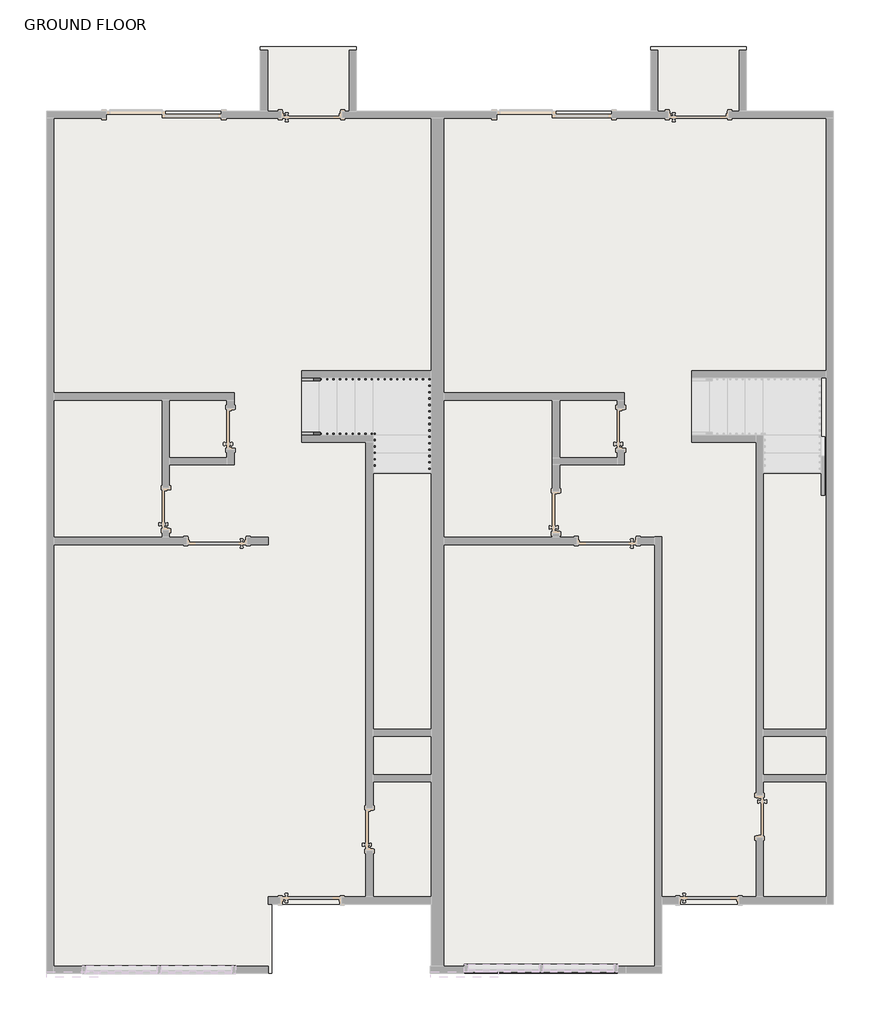
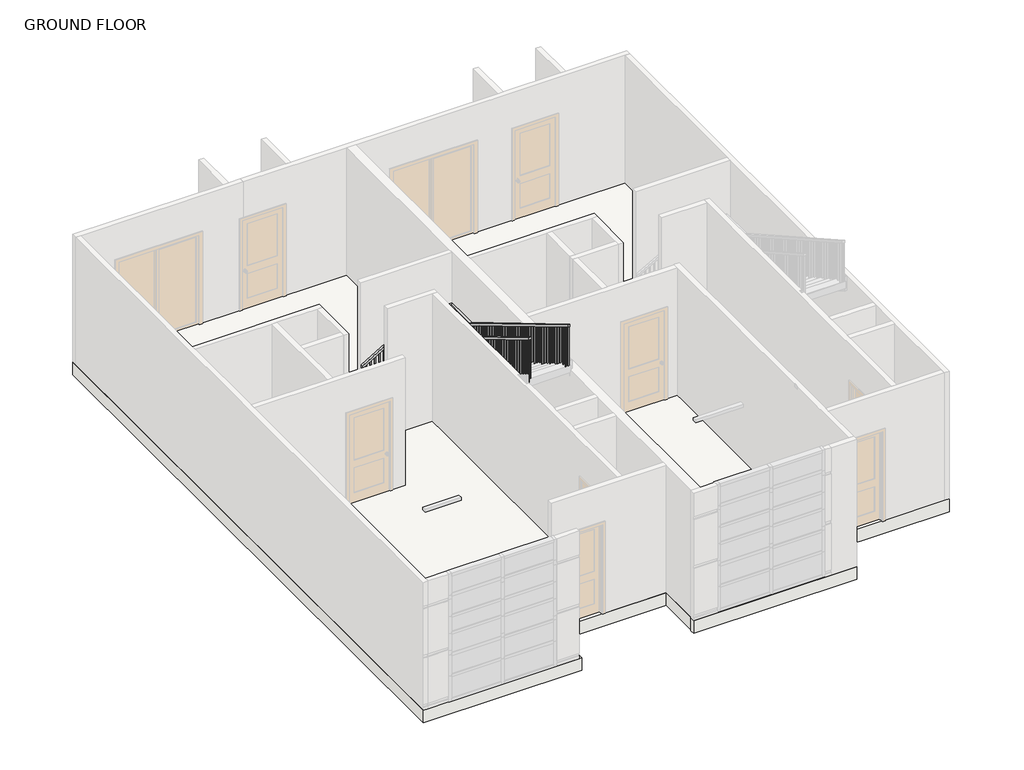
# One storey, part 3 of 4: 2 railings, 1 slab.
"""IFC4 building model written with IfcOpenShell, lengths in millimetres."""

from ifc_helpers import new_model, si_unit, frame, origin, origin_with_axes, place, context, project, spatial, polyline, outline, extrude, faceted_brep, element, save

model = new_model("IFC4")

# Units and contexts
model_context = context("Model", 3, world=origin())
ifc_project = project(units=[si_unit("LENGTHUNIT", "METRE", prefix="MILLI")], contexts=[model_context])

# Site, building, storey
site = spatial("IfcSite", under=ifc_project)
building = spatial("IfcBuilding", under=site)
storey = spatial("IfcBuildingStorey", under=building, Name="GROUND FLOOR", Elevation=304.8)

# Railings
placement = place(None, origin())
element("IfcRailing", 1, ObjectType="Handrail - Rectangular", at=placement, inside=storey, context=model_context, shape_type="SolidModel", body=[
    faceted_brep([(-14204.9595293, 3180.9909199, 1388.5333333), (-14204.9595293, 3180.9909199, 1329.3896038), (-14204.9595293, 3130.1909199, 1329.3896038), (-14204.9595293, 3130.1909199, 1388.5333333), (-13145.1007021, 3180.9909199, 2020.4352165), (-13094.3007021, 3180.9909199, 1991.5791204), (-13094.3007021, 3130.1909199, 1991.5791204), (-13145.1007021, 3130.1909199, 2020.4352165), (-13145.1007021, 3180.9909199, 2280.5581164), (-13094.3007021, 3180.9909199, 2229.7581164), (-13094.3007021, 3130.1909199, 2229.7581164), (-13145.1007021, 3130.1909199, 2280.5581164), (-13018.1007021, 3180.9909199, 2280.5581164), (-13018.1007021, 3180.9909199, 2229.7581164), (-13068.9007021, 3130.1909199, 2229.7581164), (-13068.9007021, 3130.1909199, 2280.5581164), (-13018.1007021, 3053.9909199, 2280.5581164), (-13018.1007021, 3040.0157902, 2229.7581164), (-13068.9007021, 3040.0157902, 2229.7581164), (-13068.9007021, 3053.9909199, 2280.5581164), (-13018.1007021, -567.9697052, 4436.5333333), (-13068.9007021, -567.9697052, 4436.5333333), (-13068.9007021, -567.9697052, 4377.4146252), (-13018.1007021, -567.9697052, 4377.4146252)], [[[0, 1, 2, 3]], [[1, 0, 4, 5]], [[2, 1, 5, 6]], [[3, 2, 6, 7]], [[0, 3, 7, 4]], [[5, 4, 8, 9]], [[6, 5, 9, 10]], [[7, 6, 10, 11]], [[4, 7, 11, 8]], [[9, 8, 12, 13]], [[10, 9, 13, 14]], [[11, 10, 14, 15]], [[8, 11, 15, 12]], [[13, 12, 16, 17]], [[14, 13, 17, 18]], [[15, 14, 18, 19]], [[12, 15, 19, 16]], [[20, 21, 22, 23]], [[17, 16, 20, 23]], [[18, 17, 23, 22]], [[19, 18, 22, 21]], [[16, 19, 21, 20]]]),
    extrude(outline(polyline([(-511.5340801, 4343.7849256), (-492.4840801, 4332.4453965), (-492.4840801, 3352.8), (-511.5340801, 3352.8), (-511.5340801, 4343.7849256)])), frame((-13053.0257021, 0.0, 0.0), z_axis=(1.0, 0.0, 0.0), x_axis=(0.0, 1.0, 0.0)), (0.0, 0.0, 1.0), 19.05),
    extrude(outline(polyline([(-409.9340801, 4283.3074371), (-390.8840801, 4271.967908), (-390.8840801, 3352.8), (-409.9340801, 3352.8), (-409.9340801, 4283.3074371)])), frame((-13053.0257021, 0.0, 0.0), z_axis=(1.0, 0.0, 0.0), x_axis=(0.0, 1.0, 0.0)), (0.0, 0.0, 1.0), 19.05),
    extrude(outline(polyline([(-308.3340801, 4222.8299486), (-289.2840801, 4211.4904195), (-289.2840801, 3352.8), (-308.3340801, 3352.8), (-308.3340801, 4222.8299486)])), frame((-13053.0257021, 0.0, 0.0), z_axis=(1.0, 0.0, 0.0), x_axis=(0.0, 1.0, 0.0)), (0.0, 0.0, 1.0), 19.05),
    extrude(outline(polyline([(-206.7340801, 4162.3524601), (-187.6840801, 4151.012931), (-187.6840801, 3183.4666667), (-206.7340801, 3183.4666667), (-206.7340801, 4162.3524601)])), frame((-13053.0257021, 0.0, 0.0), z_axis=(1.0, 0.0, 0.0), x_axis=(0.0, 1.0, 0.0)), (0.0, 0.0, 1.0), 19.05),
    extrude(outline(polyline([(-105.1340801, 4101.8749716), (-86.0840801, 4090.5354425), (-86.0840801, 3183.4666667), (-105.1340801, 3183.4666667), (-105.1340801, 4101.8749716)])), frame((-13053.0257021, 0.0, 0.0), z_axis=(1.0, 0.0, 0.0), x_axis=(0.0, 1.0, 0.0)), (0.0, 0.0, 1.0), 19.05),
    extrude(outline(polyline([(-3.5340801, 4041.3974831), (15.5159199, 4030.057954), (15.5159199, 3014.1333333), (-3.5340801, 3014.1333333), (-3.5340801, 4041.3974831)])), frame((-13053.0257021, 0.0, 0.0), z_axis=(1.0, 0.0, 0.0), x_axis=(0.0, 1.0, 0.0)), (0.0, 0.0, 1.0), 19.05),
    extrude(outline(polyline([(98.0659199, 3980.9199946), (117.1159199, 3969.5804655), (117.1159199, 3014.1333333), (98.0659199, 3014.1333333), (98.0659199, 3980.9199946)])), frame((-13053.0257021, 0.0, 0.0), z_axis=(1.0, 0.0, 0.0), x_axis=(0.0, 1.0, 0.0)), (0.0, 0.0, 1.0), 19.05),
    extrude(outline(polyline([(199.6659199, 3920.4425061), (218.7159199, 3909.102977), (218.7159199, 3014.1333333), (199.6659199, 3014.1333333), (199.6659199, 3920.4425061)])), frame((-13053.0257021, 0.0, 0.0), z_axis=(1.0, 0.0, 0.0), x_axis=(0.0, 1.0, 0.0)), (0.0, 0.0, 1.0), 19.05),
    extrude(outline(polyline([(301.2659199, 3859.9831899), (320.3159199, 3848.6436608), (320.3159199, 2844.8), (301.2659199, 2844.8), (301.2659199, 3859.9831899)])), frame((-13053.0257021, 0.0, 0.0), z_axis=(1.0, 0.0, 0.0), x_axis=(0.0, 1.0, 0.0)), (0.0, 0.0, 1.0), 19.05),
    extrude(outline(polyline([(402.8659199, 3799.5057014), (421.9159199, 3788.1661723), (421.9159199, 2844.8), (402.8659199, 2844.8), (402.8659199, 3799.5057014)])), frame((-13053.0257021, 0.0, 0.0), z_axis=(1.0, 0.0, 0.0), x_axis=(0.0, 1.0, 0.0)), (0.0, 0.0, 1.0), 19.05),
    extrude(outline(polyline([(504.4659199, 3739.0282129), (523.5159199, 3727.6886838), (523.5159199, 2844.8), (504.4659199, 2844.8), (504.4659199, 3739.0282129)])), frame((-13053.0257021, 0.0, 0.0), z_axis=(1.0, 0.0, 0.0), x_axis=(0.0, 1.0, 0.0)), (0.0, 0.0, 1.0), 19.05),
    extrude(outline(polyline([(606.0659199, 3678.5507244), (625.1159199, 3667.2111953), (625.1159199, 2675.4666667), (606.0659199, 2675.4666667), (606.0659199, 3678.5507244)])), frame((-13053.0257021, 0.0, 0.0), z_axis=(1.0, 0.0, 0.0), x_axis=(0.0, 1.0, 0.0)), (0.0, 0.0, 1.0), 19.05),
    extrude(outline(polyline([(707.6659199, 3618.0732359), (726.7159199, 3606.7337068), (726.7159199, 2675.4666667), (707.6659199, 2675.4666667), (707.6659199, 3618.0732359)])), frame((-13053.0257021, 0.0, 0.0), z_axis=(1.0, 0.0, 0.0), x_axis=(0.0, 1.0, 0.0)), (0.0, 0.0, 1.0), 19.05),
    extrude(outline(polyline([(809.2659199, 3557.5957474), (828.3159199, 3546.2562183), (828.3159199, 2675.4666667), (809.2659199, 2675.4666667), (809.2659199, 3557.5957474)])), frame((-13053.0257021, 0.0, 0.0), z_axis=(1.0, 0.0, 0.0), x_axis=(0.0, 1.0, 0.0)), (0.0, 0.0, 1.0), 19.05),
    extrude(outline(polyline([(910.8659199, 3497.1182589), (929.9159199, 3485.7787298), (929.9159199, 2506.1333333), (910.8659199, 2506.1333333), (910.8659199, 3497.1182589)])), frame((-13053.0257021, 0.0, 0.0), z_axis=(1.0, 0.0, 0.0), x_axis=(0.0, 1.0, 0.0)), (0.0, 0.0, 1.0), 19.05),
    extrude(outline(polyline([(1012.4659199, 3436.6407704), (1031.5159199, 3425.3012413), (1031.5159199, 2506.1333333), (1012.4659199, 2506.1333333), (1012.4659199, 3436.6407704)])), frame((-13053.0257021, 0.0, 0.0), z_axis=(1.0, 0.0, 0.0), x_axis=(0.0, 1.0, 0.0)), (0.0, 0.0, 1.0), 19.05),
    extrude(outline(polyline([(1114.0659199, 3376.1632819), (1133.1159199, 3364.8237528), (1133.1159199, 2506.1333333), (1114.0659199, 2506.1333333), (1114.0659199, 3376.1632819)])), frame((-13053.0257021, 0.0, 0.0), z_axis=(1.0, 0.0, 0.0), x_axis=(0.0, 1.0, 0.0)), (0.0, 0.0, 1.0), 19.05),
    extrude(outline(polyline([(1215.6659199, 3315.6857934), (1234.7159199, 3304.3462643), (1234.7159199, 2336.8), (1215.6659199, 2336.8), (1215.6659199, 3315.6857934)])), frame((-13053.0257021, 0.0, 0.0), z_axis=(1.0, 0.0, 0.0), x_axis=(0.0, 1.0, 0.0)), (0.0, 0.0, 1.0), 19.05),
    extrude(outline(polyline([(1317.2659199, 3255.2083049), (1336.3159199, 3243.8687758), (1336.3159199, 2336.8), (1317.2659199, 2336.8), (1317.2659199, 3255.2083049)])), frame((-13053.0257021, 0.0, 0.0), z_axis=(1.0, 0.0, 0.0), x_axis=(0.0, 1.0, 0.0)), (0.0, 0.0, 1.0), 19.05),
    extrude(outline(polyline([(1418.8659199, 3194.7308164), (1437.9159199, 3183.3912873), (1437.9159199, 2167.4666667), (1418.8659199, 2167.4666667), (1418.8659199, 3194.7308164)])), frame((-13053.0257021, 0.0, 0.0), z_axis=(1.0, 0.0, 0.0), x_axis=(0.0, 1.0, 0.0)), (0.0, 0.0, 1.0), 19.05),
    extrude(outline(polyline([(1520.4659199, 3134.2533279), (1539.5159199, 3122.9137988), (1539.5159199, 2167.4666667), (1520.4659199, 2167.4666667), (1520.4659199, 3134.2533279)])), frame((-13053.0257021, 0.0, 0.0), z_axis=(1.0, 0.0, 0.0), x_axis=(0.0, 1.0, 0.0)), (0.0, 0.0, 1.0), 19.05),
    extrude(outline(polyline([(1622.0659199, 3073.7758394), (1641.1159199, 3062.4363103), (1641.1159199, 2167.4666667), (1622.0659199, 2167.4666667), (1622.0659199, 3073.7758394)])), frame((-13053.0257021, 0.0, 0.0), z_axis=(1.0, 0.0, 0.0), x_axis=(0.0, 1.0, 0.0)), (0.0, 0.0, 1.0), 19.05),
    extrude(outline(polyline([(1723.6659199, 3013.3165232), (1742.7159199, 3001.9769941), (1742.7159199, 1998.1333333), (1723.6659199, 1998.1333333), (1723.6659199, 3013.3165232)])), frame((-13053.0257021, 0.0, 0.0), z_axis=(1.0, 0.0, 0.0), x_axis=(0.0, 1.0, 0.0)), (0.0, 0.0, 1.0), 19.05),
    extrude(outline(polyline([(1825.2659199, 2952.8390347), (1844.3159199, 2941.4995057), (1844.3159199, 1998.1333333), (1825.2659199, 1998.1333333), (1825.2659199, 2952.8390347)])), frame((-13053.0257021, 0.0, 0.0), z_axis=(1.0, 0.0, 0.0), x_axis=(0.0, 1.0, 0.0)), (0.0, 0.0, 1.0), 19.05),
    extrude(outline(polyline([(1926.8659199, 2892.3615462), (1945.9159199, 2881.0220172), (1945.9159199, 1998.1333333), (1926.8659199, 1998.1333333), (1926.8659199, 2892.3615462)])), frame((-13053.0257021, 0.0, 0.0), z_axis=(1.0, 0.0, 0.0), x_axis=(0.0, 1.0, 0.0)), (0.0, 0.0, 1.0), 19.05),
    extrude(outline(polyline([(2028.4659199, 2831.8840577), (2047.5159199, 2820.5445287), (2047.5159199, 1828.8), (2028.4659199, 1828.8), (2028.4659199, 2831.8840577)])), frame((-13053.0257021, 0.0, 0.0), z_axis=(1.0, 0.0, 0.0), x_axis=(0.0, 1.0, 0.0)), (0.0, 0.0, 1.0), 19.05),
    extrude(outline(polyline([(2130.0659199, 2771.4065692), (2149.1159199, 2760.0670402), (2149.1159199, 1828.8), (2130.0659199, 1828.8), (2130.0659199, 2771.4065692)])), frame((-13053.0257021, 0.0, 0.0), z_axis=(1.0, 0.0, 0.0), x_axis=(0.0, 1.0, 0.0)), (0.0, 0.0, 1.0), 19.05),
    extrude(outline(polyline([(2231.6659199, 2710.9290808), (2250.7159199, 2699.5895517), (2250.7159199, 1828.8), (2231.6659199, 1828.8), (2231.6659199, 2710.9290808)])), frame((-13053.0257021, 0.0, 0.0), z_axis=(1.0, 0.0, 0.0), x_axis=(0.0, 1.0, 0.0)), (0.0, 0.0, 1.0), 19.05),
    extrude(outline(polyline([(2333.2659199, 2650.4515923), (2352.3159199, 2639.1120632), (2352.3159199, 1659.4666667), (2333.2659199, 1659.4666667), (2333.2659199, 2650.4515923)])), frame((-13053.0257021, 0.0, 0.0), z_axis=(1.0, 0.0, 0.0), x_axis=(0.0, 1.0, 0.0)), (0.0, 0.0, 1.0), 19.05),
    extrude(outline(polyline([(2434.8659199, 2589.9741038), (2453.9159199, 2578.6345747), (2453.9159199, 1659.4666667), (2434.8659199, 1659.4666667), (2434.8659199, 2589.9741038)])), frame((-13053.0257021, 0.0, 0.0), z_axis=(1.0, 0.0, 0.0), x_axis=(0.0, 1.0, 0.0)), (0.0, 0.0, 1.0), 19.05),
    extrude(outline(polyline([(2536.4659199, 2529.4966153), (2555.5159199, 2518.1570862), (2555.5159199, 1659.4666667), (2536.4659199, 1659.4666667), (2536.4659199, 2529.4966153)])), frame((-13053.0257021, 0.0, 0.0), z_axis=(1.0, 0.0, 0.0), x_axis=(0.0, 1.0, 0.0)), (0.0, 0.0, 1.0), 19.05),
    extrude(outline(polyline([(2638.0659199, 2469.0191268), (2657.1159199, 2457.6795977), (2657.1159199, 1490.1333333), (2638.0659199, 1490.1333333), (2638.0659199, 2469.0191268)])), frame((-13053.0257021, 0.0, 0.0), z_axis=(1.0, 0.0, 0.0), x_axis=(0.0, 1.0, 0.0)), (0.0, 0.0, 1.0), 19.05),
    extrude(outline(polyline([(2739.6659199, 2408.5416383), (2758.7159199, 2397.2021092), (2758.7159199, 1490.1333333), (2739.6659199, 1490.1333333), (2739.6659199, 2408.5416383)])), frame((-13053.0257021, 0.0, 0.0), z_axis=(1.0, 0.0, 0.0), x_axis=(0.0, 1.0, 0.0)), (0.0, 0.0, 1.0), 19.05),
    extrude(outline(polyline([(2841.2659199, 2348.0641498), (2860.3159199, 2336.7246207), (2860.3159199, 1320.8), (2841.2659199, 1320.8), (2841.2659199, 2348.0641498)])), frame((-13053.0257021, 0.0, 0.0), z_axis=(1.0, 0.0, 0.0), x_axis=(0.0, 1.0, 0.0)), (0.0, 0.0, 1.0), 19.05),
    extrude(outline(polyline([(2942.8659199, 2287.5866613), (2961.9159199, 2276.2471322), (2961.9159199, 1320.8), (2942.8659199, 1320.8), (2942.8659199, 2287.5866613)])), frame((-13053.0257021, 0.0, 0.0), z_axis=(1.0, 0.0, 0.0), x_axis=(0.0, 1.0, 0.0)), (0.0, 0.0, 1.0), 19.05),
    extrude(outline(polyline([(3044.4659199, 2227.1091728), (3063.5159199, 2215.7696437), (3063.5159199, 1320.8), (3044.4659199, 1320.8), (3044.4659199, 2227.1091728)])), frame((-13053.0257021, 0.0, 0.0), z_axis=(1.0, 0.0, 0.0), x_axis=(0.0, 1.0, 0.0)), (0.0, 0.0, 1.0), 19.05),
    extrude(outline(polyline([(-13096.8845293, 3146.0659199), (-13096.8845293, 3165.1159199), (-13077.8345293, 3165.1159199), (-13077.8345293, 3146.0659199), (-13096.8845293, 3146.0659199)])), frame((0.0, 0.0, 982.1333333), z_axis=(0.0, 0.0, 1.0), x_axis=(1.0, 0.0, 0.0)), (0.0, 0.0, 1.0), 1247.624783),
    extrude(outline(polyline([(1940.821204, -13179.4345293), (1929.4633415, -13198.4845293), (982.1333333, -13198.4845293), (982.1333333, -13179.4345293), (1940.821204, -13179.4345293)])), frame((0.0, 3146.0659199, 0.0), z_axis=(0.0, 1.0, 0.0), x_axis=(0.0, 0.0, 1.0)), (0.0, 0.0, 1.0), 19.05),
    extrude(outline(polyline([(1880.2459371, -13281.0345293), (1868.8880746, -13300.0845293), (982.1333333, -13300.0845293), (982.1333333, -13281.0345293), (1880.2459371, -13281.0345293)])), frame((0.0, 3146.0659199, 0.0), z_axis=(0.0, 1.0, 0.0), x_axis=(0.0, 0.0, 1.0)), (0.0, 0.0, 1.0), 19.05),
    extrude(outline(polyline([(1819.6706702, -13382.6345293), (1808.3128077, -13401.6845293), (812.8, -13401.6845293), (812.8, -13382.6345293), (1819.6706702, -13382.6345293)])), frame((0.0, 3146.0659199, 0.0), z_axis=(0.0, 1.0, 0.0), x_axis=(0.0, 0.0, 1.0)), (0.0, 0.0, 1.0), 19.05),
    extrude(outline(polyline([(1759.0954033, -13484.2345293), (1747.7375408, -13503.2845293), (812.8, -13503.2845293), (812.8, -13484.2345293), (1759.0954033, -13484.2345293)])), frame((0.0, 3146.0659199, 0.0), z_axis=(0.0, 1.0, 0.0), x_axis=(0.0, 0.0, 1.0)), (0.0, 0.0, 1.0), 19.05),
    extrude(outline(polyline([(1698.5201365, -13585.8345293), (1687.1622739, -13604.8845293), (812.8, -13604.8845293), (812.8, -13585.8345293), (1698.5201365, -13585.8345293)])), frame((0.0, 3146.0659199, 0.0), z_axis=(0.0, 1.0, 0.0), x_axis=(0.0, 0.0, 1.0)), (0.0, 0.0, 1.0), 19.05),
    extrude(outline(polyline([(1637.9448696, -13687.4345293), (1626.587007, -13706.4845293), (643.4666667, -13706.4845293), (643.4666667, -13687.4345293), (1637.9448696, -13687.4345293)])), frame((0.0, 3146.0659199, 0.0), z_axis=(0.0, 1.0, 0.0), x_axis=(0.0, 0.0, 1.0)), (0.0, 0.0, 1.0), 19.05),
    extrude(outline(polyline([(1577.3696027, -13789.0345293), (1566.0117401, -13808.0845293), (643.4666667, -13808.0845293), (643.4666667, -13789.0345293), (1577.3696027, -13789.0345293)])), frame((0.0, 3146.0659199, 0.0), z_axis=(0.0, 1.0, 0.0), x_axis=(0.0, 0.0, 1.0)), (0.0, 0.0, 1.0), 19.05),
    extrude(outline(polyline([(1516.7943358, -13890.6345293), (1505.4364732, -13909.6845293), (643.4666667, -13909.6845293), (643.4666667, -13890.6345293), (1516.7943358, -13890.6345293)])), frame((0.0, 3146.0659199, 0.0), z_axis=(0.0, 1.0, 0.0), x_axis=(0.0, 0.0, 1.0)), (0.0, 0.0, 1.0), 19.05),
    extrude(outline(polyline([(1456.2190689, -13992.2345293), (1444.8612063, -14011.2845293), (474.1333333, -14011.2845293), (474.1333333, -13992.2345293), (1456.2190689, -13992.2345293)])), frame((0.0, 3146.0659199, 0.0), z_axis=(0.0, 1.0, 0.0), x_axis=(0.0, 0.0, 1.0)), (0.0, 0.0, 1.0), 19.05),
    extrude(outline(polyline([(1395.643802, -14093.8345293), (1384.2859394, -14112.8845293), (474.1333333, -14112.8845293), (474.1333333, -14093.8345293), (1395.643802, -14093.8345293)])), frame((0.0, 3146.0659199, 0.0), z_axis=(0.0, 1.0, 0.0), x_axis=(0.0, 0.0, 1.0)), (0.0, 0.0, 1.0), 19.05),
    extrude(outline(polyline([(-13053.0257021, 3146.0659199), (-13053.0257021, 3165.1159199), (-13033.9757021, 3165.1159199), (-13033.9757021, 3146.0659199), (-13053.0257021, 3146.0659199)])), frame((0.0, 0.0, 1151.4666667), z_axis=(0.0, 0.0, 1.0), x_axis=(1.0, 0.0, 0.0)), (0.0, 0.0, 1.0), 1078.2914497),
    extrude(outline(polyline([(-567.9697052, 4377.4146252), (-548.9197052, 4366.0750961), (-548.9197052, 3352.8), (-567.9697052, 3352.8), (-567.9697052, 4377.4146252)])), frame((-13053.0257021, 0.0, 0.0), z_axis=(1.0, 0.0, 0.0), x_axis=(0.0, 1.0, 0.0)), (0.0, 0.0, 1.0), 19.05),
    extrude(outline(polyline([(1340.7474664, -14185.9095293), (1329.3896038, -14204.9595293), (474.1333333, -14204.9595293), (474.1333333, -14185.9095293), (1340.7474664, -14185.9095293)])), frame((0.0, 3146.0659199, 0.0), z_axis=(0.0, 1.0, 0.0), x_axis=(0.0, 0.0, 1.0)), (0.0, 0.0, 1.0), 19.05),
])
element("IfcRailing", 2, ObjectType="Handrail - Rectangular", at=placement, inside=storey, context=model_context, shape_type="SolidModel", body=[
    faceted_brep([(-14204.9595293, 4044.5909199, 1388.5333333), (-14204.9595293, 4044.5909199, 1329.3896038), (-14204.9595293, 3993.7909199, 1329.3896038), (-14204.9595293, 3993.7909199, 1388.5333333), (-12920.7685518, 4044.5909199, 2154.1850185), (-12906.774013, 4044.5909199, 2103.3850185), (-12906.774013, 3993.7909199, 2103.3850185), (-12920.7685518, 3993.7909199, 2154.1850185), (-12143.6860997, 4044.5909199, 2154.1850185), (-12143.6860997, 4044.5909199, 2103.3850185), (-12194.4860997, 3993.7909199, 2103.3850185), (-12194.4860997, 3993.7909199, 2154.1850185), (-12143.6860997, 3266.2931677, 2154.1850185), (-12143.6860997, 3252.3180379, 2103.3850185), (-12194.4860997, 3252.3180379, 2103.3850185), (-12194.4860997, 3266.2931677, 2154.1850185), (-12143.6860997, -567.9697052, 4436.5333333), (-12194.4860997, -567.9697052, 4436.5333333), (-12194.4860997, -567.9697052, 4377.4146252), (-12143.6860997, -567.9697052, 4377.4146252)], [[[0, 1, 2, 3]], [[1, 0, 4, 5]], [[2, 1, 5, 6]], [[3, 2, 6, 7]], [[0, 3, 7, 4]], [[5, 4, 8, 9]], [[6, 5, 9, 10]], [[7, 6, 10, 11]], [[4, 7, 11, 8]], [[9, 8, 12, 13]], [[10, 9, 13, 14]], [[11, 10, 14, 15]], [[8, 11, 15, 12]], [[16, 17, 18, 19]], [[13, 12, 16, 19]], [[14, 13, 19, 18]], [[15, 14, 18, 17]], [[12, 15, 17, 16]]]),
    extrude(outline(polyline([(-543.2840801, 4362.6841407), (-543.2840801, 3352.8), (-562.3340801, 3352.8), (-562.3340801, 4374.0236698), (-543.2840801, 4362.6841407)])), frame((-12178.6110997, 0.0, 0.0), z_axis=(1.0, 0.0, 0.0), x_axis=(0.0, 1.0, 0.0)), (0.0, 0.0, 1.0), 19.05),
    extrude(outline(polyline([(-441.6840801, 4302.2066522), (-441.6840801, 3352.8), (-460.7340801, 3352.8), (-460.7340801, 4313.5461813), (-441.6840801, 4302.2066522)])), frame((-12178.6110997, 0.0, 0.0), z_axis=(1.0, 0.0, 0.0), x_axis=(0.0, 1.0, 0.0)), (0.0, 0.0, 1.0), 19.05),
    extrude(outline(polyline([(-340.0840801, 4241.7291637), (-340.0840801, 3352.8), (-359.1340801, 3352.8), (-359.1340801, 4253.0686928), (-340.0840801, 4241.7291637)])), frame((-12178.6110997, 0.0, 0.0), z_axis=(1.0, 0.0, 0.0), x_axis=(0.0, 1.0, 0.0)), (0.0, 0.0, 1.0), 19.05),
    extrude(outline(polyline([(-238.4840801, 4181.2516752), (-238.4840801, 3183.4666667), (-257.5340801, 3183.4666667), (-257.5340801, 4192.5912043), (-238.4840801, 4181.2516752)])), frame((-12178.6110997, 0.0, 0.0), z_axis=(1.0, 0.0, 0.0), x_axis=(0.0, 1.0, 0.0)), (0.0, 0.0, 1.0), 19.05),
    extrude(outline(polyline([(-136.8840801, 4120.7741868), (-136.8840801, 3183.4666667), (-155.9340801, 3183.4666667), (-155.9340801, 4132.1137158), (-136.8840801, 4120.7741868)])), frame((-12178.6110997, 0.0, 0.0), z_axis=(1.0, 0.0, 0.0), x_axis=(0.0, 1.0, 0.0)), (0.0, 0.0, 1.0), 19.05),
    extrude(outline(polyline([(-35.2840801, 4060.2966983), (-35.2840801, 3183.4666667), (-54.3340801, 3183.4666667), (-54.3340801, 4071.6362273), (-35.2840801, 4060.2966983)])), frame((-12178.6110997, 0.0, 0.0), z_axis=(1.0, 0.0, 0.0), x_axis=(0.0, 1.0, 0.0)), (0.0, 0.0, 1.0), 19.05),
    extrude(outline(polyline([(66.3159199, 3999.8192098), (66.3159199, 3014.1333333), (47.2659199, 3014.1333333), (47.2659199, 4011.1587388), (66.3159199, 3999.8192098)])), frame((-12178.6110997, 0.0, 0.0), z_axis=(1.0, 0.0, 0.0), x_axis=(0.0, 1.0, 0.0)), (0.0, 0.0, 1.0), 19.05),
    extrude(outline(polyline([(167.9159199, 3939.3417213), (167.9159199, 3014.1333333), (148.8659199, 3014.1333333), (148.8659199, 3950.6812503), (167.9159199, 3939.3417213)])), frame((-12178.6110997, 0.0, 0.0), z_axis=(1.0, 0.0, 0.0), x_axis=(0.0, 1.0, 0.0)), (0.0, 0.0, 1.0), 19.05),
    extrude(outline(polyline([(269.5159199, 3878.8642328), (269.5159199, 3014.1333333), (250.4659199, 3014.1333333), (250.4659199, 3890.2037619), (269.5159199, 3878.8642328)])), frame((-12178.6110997, 0.0, 0.0), z_axis=(1.0, 0.0, 0.0), x_axis=(0.0, 1.0, 0.0)), (0.0, 0.0, 1.0), 19.05),
    extrude(outline(polyline([(371.1159199, 3818.3867443), (371.1159199, 2844.8), (352.0659199, 2844.8), (352.0659199, 3829.7262734), (371.1159199, 3818.3867443)])), frame((-12178.6110997, 0.0, 0.0), z_axis=(1.0, 0.0, 0.0), x_axis=(0.0, 1.0, 0.0)), (0.0, 0.0, 1.0), 19.05),
    extrude(outline(polyline([(472.7159199, 3757.9274281), (472.7159199, 2844.8), (453.6659199, 2844.8), (453.6659199, 3769.2669572), (472.7159199, 3757.9274281)])), frame((-12178.6110997, 0.0, 0.0), z_axis=(1.0, 0.0, 0.0), x_axis=(0.0, 1.0, 0.0)), (0.0, 0.0, 1.0), 19.05),
    extrude(outline(polyline([(574.3159199, 3697.4499396), (574.3159199, 2844.8), (555.2659199, 2844.8), (555.2659199, 3708.7894687), (574.3159199, 3697.4499396)])), frame((-12178.6110997, 0.0, 0.0), z_axis=(1.0, 0.0, 0.0), x_axis=(0.0, 1.0, 0.0)), (0.0, 0.0, 1.0), 19.05),
    extrude(outline(polyline([(675.9159199, 3636.9724511), (675.9159199, 2675.4666667), (656.8659199, 2675.4666667), (656.8659199, 3648.3119802), (675.9159199, 3636.9724511)])), frame((-12178.6110997, 0.0, 0.0), z_axis=(1.0, 0.0, 0.0), x_axis=(0.0, 1.0, 0.0)), (0.0, 0.0, 1.0), 19.05),
    extrude(outline(polyline([(777.5159199, 3576.4949626), (777.5159199, 2675.4666667), (758.4659199, 2675.4666667), (758.4659199, 3587.8344917), (777.5159199, 3576.4949626)])), frame((-12178.6110997, 0.0, 0.0), z_axis=(1.0, 0.0, 0.0), x_axis=(0.0, 1.0, 0.0)), (0.0, 0.0, 1.0), 19.05),
    extrude(outline(polyline([(879.1159199, 3516.0174741), (879.1159199, 2506.1333333), (860.0659199, 2506.1333333), (860.0659199, 3527.3570032), (879.1159199, 3516.0174741)])), frame((-12178.6110997, 0.0, 0.0), z_axis=(1.0, 0.0, 0.0), x_axis=(0.0, 1.0, 0.0)), (0.0, 0.0, 1.0), 19.05),
    extrude(outline(polyline([(980.7159199, 3455.5399856), (980.7159199, 2506.1333333), (961.6659199, 2506.1333333), (961.6659199, 3466.8795147), (980.7159199, 3455.5399856)])), frame((-12178.6110997, 0.0, 0.0), z_axis=(1.0, 0.0, 0.0), x_axis=(0.0, 1.0, 0.0)), (0.0, 0.0, 1.0), 19.05),
    extrude(outline(polyline([(1082.3159199, 3395.0624971), (1082.3159199, 2506.1333333), (1063.2659199, 2506.1333333), (1063.2659199, 3406.4020262), (1082.3159199, 3395.0624971)])), frame((-12178.6110997, 0.0, 0.0), z_axis=(1.0, 0.0, 0.0), x_axis=(0.0, 1.0, 0.0)), (0.0, 0.0, 1.0), 19.05),
    extrude(outline(polyline([(1183.9159199, 3334.5850086), (1183.9159199, 2336.8), (1164.8659199, 2336.8), (1164.8659199, 3345.9245377), (1183.9159199, 3334.5850086)])), frame((-12178.6110997, 0.0, 0.0), z_axis=(1.0, 0.0, 0.0), x_axis=(0.0, 1.0, 0.0)), (0.0, 0.0, 1.0), 19.05),
    extrude(outline(polyline([(1285.5159199, 3274.1075201), (1285.5159199, 2336.8), (1266.4659199, 2336.8), (1266.4659199, 3285.4470492), (1285.5159199, 3274.1075201)])), frame((-12178.6110997, 0.0, 0.0), z_axis=(1.0, 0.0, 0.0), x_axis=(0.0, 1.0, 0.0)), (0.0, 0.0, 1.0), 19.05),
    extrude(outline(polyline([(1387.1159199, 3213.6300316), (1387.1159199, 2336.8), (1368.0659199, 2336.8), (1368.0659199, 3224.9695607), (1387.1159199, 3213.6300316)])), frame((-12178.6110997, 0.0, 0.0), z_axis=(1.0, 0.0, 0.0), x_axis=(0.0, 1.0, 0.0)), (0.0, 0.0, 1.0), 19.05),
    extrude(outline(polyline([(1488.7159199, 3153.1525431), (1488.7159199, 2167.4666667), (1469.6659199, 2167.4666667), (1469.6659199, 3164.4920722), (1488.7159199, 3153.1525431)])), frame((-12178.6110997, 0.0, 0.0), z_axis=(1.0, 0.0, 0.0), x_axis=(0.0, 1.0, 0.0)), (0.0, 0.0, 1.0), 19.05),
    extrude(outline(polyline([(1590.3159199, 3092.6750546), (1590.3159199, 2167.4666667), (1571.2659199, 2167.4666667), (1571.2659199, 3104.0145837), (1590.3159199, 3092.6750546)])), frame((-12178.6110997, 0.0, 0.0), z_axis=(1.0, 0.0, 0.0), x_axis=(0.0, 1.0, 0.0)), (0.0, 0.0, 1.0), 19.05),
    extrude(outline(polyline([(1691.9159199, 3032.1975661), (1691.9159199, 2167.4666667), (1672.8659199, 2167.4666667), (1672.8659199, 3043.5370952), (1691.9159199, 3032.1975661)])), frame((-12178.6110997, 0.0, 0.0), z_axis=(1.0, 0.0, 0.0), x_axis=(0.0, 1.0, 0.0)), (0.0, 0.0, 1.0), 19.05),
    extrude(outline(polyline([(1793.5159199, 2971.7200776), (1793.5159199, 1998.1333333), (1774.4659199, 1998.1333333), (1774.4659199, 2983.0596067), (1793.5159199, 2971.7200776)])), frame((-12178.6110997, 0.0, 0.0), z_axis=(1.0, 0.0, 0.0), x_axis=(0.0, 1.0, 0.0)), (0.0, 0.0, 1.0), 19.05),
    extrude(outline(polyline([(1895.1159199, 2911.2607614), (1895.1159199, 1998.1333333), (1876.0659199, 1998.1333333), (1876.0659199, 2922.6002905), (1895.1159199, 2911.2607614)])), frame((-12178.6110997, 0.0, 0.0), z_axis=(1.0, 0.0, 0.0), x_axis=(0.0, 1.0, 0.0)), (0.0, 0.0, 1.0), 19.05),
    extrude(outline(polyline([(1996.7159199, 2850.7832729), (1996.7159199, 1998.1333333), (1977.6659199, 1998.1333333), (1977.6659199, 2862.122802), (1996.7159199, 2850.7832729)])), frame((-12178.6110997, 0.0, 0.0), z_axis=(1.0, 0.0, 0.0), x_axis=(0.0, 1.0, 0.0)), (0.0, 0.0, 1.0), 19.05),
    extrude(outline(polyline([(2098.3159199, 2790.3057844), (2098.3159199, 1828.8), (2079.2659199, 1828.8), (2079.2659199, 2801.6453135), (2098.3159199, 2790.3057844)])), frame((-12178.6110997, 0.0, 0.0), z_axis=(1.0, 0.0, 0.0), x_axis=(0.0, 1.0, 0.0)), (0.0, 0.0, 1.0), 19.05),
    extrude(outline(polyline([(2199.9159199, 2729.8282959), (2199.9159199, 1828.8), (2180.8659199, 1828.8), (2180.8659199, 2741.167825), (2199.9159199, 2729.8282959)])), frame((-12178.6110997, 0.0, 0.0), z_axis=(1.0, 0.0, 0.0), x_axis=(0.0, 1.0, 0.0)), (0.0, 0.0, 1.0), 19.05),
    extrude(outline(polyline([(2301.5159199, 2669.3508074), (2301.5159199, 1659.4666667), (2282.4659199, 1659.4666667), (2282.4659199, 2680.6903365), (2301.5159199, 2669.3508074)])), frame((-12178.6110997, 0.0, 0.0), z_axis=(1.0, 0.0, 0.0), x_axis=(0.0, 1.0, 0.0)), (0.0, 0.0, 1.0), 19.05),
    extrude(outline(polyline([(2403.1159199, 2608.8733189), (2403.1159199, 1659.4666667), (2384.0659199, 1659.4666667), (2384.0659199, 2620.212848), (2403.1159199, 2608.8733189)])), frame((-12178.6110997, 0.0, 0.0), z_axis=(1.0, 0.0, 0.0), x_axis=(0.0, 1.0, 0.0)), (0.0, 0.0, 1.0), 19.05),
    extrude(outline(polyline([(2504.7159199, 2548.3958304), (2504.7159199, 1659.4666667), (2485.6659199, 1659.4666667), (2485.6659199, 2559.7353595), (2504.7159199, 2548.3958304)])), frame((-12178.6110997, 0.0, 0.0), z_axis=(1.0, 0.0, 0.0), x_axis=(0.0, 1.0, 0.0)), (0.0, 0.0, 1.0), 19.05),
    extrude(outline(polyline([(2606.3159199, 2487.9183419), (2606.3159199, 1490.1333333), (2587.2659199, 1490.1333333), (2587.2659199, 2499.257871), (2606.3159199, 2487.9183419)])), frame((-12178.6110997, 0.0, 0.0), z_axis=(1.0, 0.0, 0.0), x_axis=(0.0, 1.0, 0.0)), (0.0, 0.0, 1.0), 19.05),
    extrude(outline(polyline([(2707.9159199, 2427.4408534), (2707.9159199, 1490.1333333), (2688.8659199, 1490.1333333), (2688.8659199, 2438.7803825), (2707.9159199, 2427.4408534)])), frame((-12178.6110997, 0.0, 0.0), z_axis=(1.0, 0.0, 0.0), x_axis=(0.0, 1.0, 0.0)), (0.0, 0.0, 1.0), 19.05),
    extrude(outline(polyline([(2809.5159199, 2366.9633649), (2809.5159199, 1490.1333333), (2790.4659199, 1490.1333333), (2790.4659199, 2378.302894), (2809.5159199, 2366.9633649)])), frame((-12178.6110997, 0.0, 0.0), z_axis=(1.0, 0.0, 0.0), x_axis=(0.0, 1.0, 0.0)), (0.0, 0.0, 1.0), 19.05),
    extrude(outline(polyline([(2911.1159199, 2306.4858764), (2911.1159199, 1320.8), (2892.0659199, 1320.8), (2892.0659199, 2317.8254055), (2911.1159199, 2306.4858764)])), frame((-12178.6110997, 0.0, 0.0), z_axis=(1.0, 0.0, 0.0), x_axis=(0.0, 1.0, 0.0)), (0.0, 0.0, 1.0), 19.05),
    extrude(outline(polyline([(3012.7159199, 2246.0083879), (3012.7159199, 1320.8), (2993.6659199, 1320.8), (2993.6659199, 2257.347917), (3012.7159199, 2246.0083879)])), frame((-12178.6110997, 0.0, 0.0), z_axis=(1.0, 0.0, 0.0), x_axis=(0.0, 1.0, 0.0)), (0.0, 0.0, 1.0), 19.05),
    extrude(outline(polyline([(3114.3159199, 2185.5308994), (3114.3159199, 1320.8), (3095.2659199, 1320.8), (3095.2659199, 2196.8704285), (3114.3159199, 2185.5308994)])), frame((-12178.6110997, 0.0, 0.0), z_axis=(1.0, 0.0, 0.0), x_axis=(0.0, 1.0, 0.0)), (0.0, 0.0, 1.0), 19.05),
    extrude(outline(polyline([(3215.9159199, 2125.0534109), (3215.9159199, 1151.4666667), (3196.8659199, 1151.4666667), (3196.8659199, 2136.39294), (3215.9159199, 2125.0534109)])), frame((-12178.6110997, 0.0, 0.0), z_axis=(1.0, 0.0, 0.0), x_axis=(0.0, 1.0, 0.0)), (0.0, 0.0, 1.0), 19.05),
    extrude(outline(polyline([(-12159.5610997, 3317.5159199), (-12159.5610997, 3298.4659199), (-12178.6110997, 3298.4659199), (-12178.6110997, 3317.5159199), (-12159.5610997, 3317.5159199)])), frame((0.0, 0.0, 1151.4666667), z_axis=(0.0, 0.0, 1.0), x_axis=(1.0, 0.0, 0.0)), (0.0, 0.0, 1.0), 951.9183518),
    extrude(outline(polyline([(-12159.5610997, 3419.1159199), (-12159.5610997, 3400.0659199), (-12178.6110997, 3400.0659199), (-12178.6110997, 3419.1159199), (-12159.5610997, 3419.1159199)])), frame((0.0, 0.0, 1151.4666667), z_axis=(0.0, 0.0, 1.0), x_axis=(1.0, 0.0, 0.0)), (0.0, 0.0, 1.0), 951.9183518),
    extrude(outline(polyline([(-12159.5610997, 3520.7159199), (-12159.5610997, 3501.6659199), (-12178.6110997, 3501.6659199), (-12178.6110997, 3520.7159199), (-12159.5610997, 3520.7159199)])), frame((0.0, 0.0, 1151.4666667), z_axis=(0.0, 0.0, 1.0), x_axis=(1.0, 0.0, 0.0)), (0.0, 0.0, 1.0), 951.9183518),
    extrude(outline(polyline([(-12159.5610997, 3622.3159199), (-12159.5610997, 3603.2659199), (-12178.6110997, 3603.2659199), (-12178.6110997, 3622.3159199), (-12159.5610997, 3622.3159199)])), frame((0.0, 0.0, 1151.4666667), z_axis=(0.0, 0.0, 1.0), x_axis=(1.0, 0.0, 0.0)), (0.0, 0.0, 1.0), 951.9183518),
    extrude(outline(polyline([(-12159.5610997, 3723.9159199), (-12159.5610997, 3704.8659199), (-12178.6110997, 3704.8659199), (-12178.6110997, 3723.9159199), (-12159.5610997, 3723.9159199)])), frame((0.0, 0.0, 1151.4666667), z_axis=(0.0, 0.0, 1.0), x_axis=(1.0, 0.0, 0.0)), (0.0, 0.0, 1.0), 951.9183518),
    extrude(outline(polyline([(-12159.5610997, 3825.5159199), (-12159.5610997, 3806.4659199), (-12178.6110997, 3806.4659199), (-12178.6110997, 3825.5159199), (-12159.5610997, 3825.5159199)])), frame((0.0, 0.0, 1151.4666667), z_axis=(0.0, 0.0, 1.0), x_axis=(1.0, 0.0, 0.0)), (0.0, 0.0, 1.0), 951.9183518),
    extrude(outline(polyline([(-12159.5610997, 3927.1159199), (-12159.5610997, 3908.0659199), (-12178.6110997, 3908.0659199), (-12178.6110997, 3927.1159199), (-12159.5610997, 3927.1159199)])), frame((0.0, 0.0, 1151.4666667), z_axis=(0.0, 0.0, 1.0), x_axis=(1.0, 0.0, 0.0)), (0.0, 0.0, 1.0), 951.9183518),
    extrude(outline(polyline([(-12182.4845293, 4028.7159199), (-12163.4345293, 4028.7159199), (-12163.4345293, 4009.6659199), (-12182.4845293, 4009.6659199), (-12182.4845293, 4028.7159199)])), frame((0.0, 0.0, 1151.4666667), z_axis=(0.0, 0.0, 1.0), x_axis=(1.0, 0.0, 0.0)), (0.0, 0.0, 1.0), 951.9183518),
    extrude(outline(polyline([(-12284.0845293, 4028.7159199), (-12265.0345293, 4028.7159199), (-12265.0345293, 4009.6659199), (-12284.0845293, 4009.6659199), (-12284.0845293, 4028.7159199)])), frame((0.0, 0.0, 1151.4666667), z_axis=(0.0, 0.0, 1.0), x_axis=(1.0, 0.0, 0.0)), (0.0, 0.0, 1.0), 951.9183518),
    extrude(outline(polyline([(-12385.6845293, 4028.7159199), (-12366.6345293, 4028.7159199), (-12366.6345293, 4009.6659199), (-12385.6845293, 4009.6659199), (-12385.6845293, 4028.7159199)])), frame((0.0, 0.0, 1151.4666667), z_axis=(0.0, 0.0, 1.0), x_axis=(1.0, 0.0, 0.0)), (0.0, 0.0, 1.0), 951.9183518),
    extrude(outline(polyline([(-12487.2845293, 4028.7159199), (-12468.2345293, 4028.7159199), (-12468.2345293, 4009.6659199), (-12487.2845293, 4009.6659199), (-12487.2845293, 4028.7159199)])), frame((0.0, 0.0, 1151.4666667), z_axis=(0.0, 0.0, 1.0), x_axis=(1.0, 0.0, 0.0)), (0.0, 0.0, 1.0), 951.9183518),
    extrude(outline(polyline([(-12588.8845293, 4028.7159199), (-12569.8345293, 4028.7159199), (-12569.8345293, 4009.6659199), (-12588.8845293, 4009.6659199), (-12588.8845293, 4028.7159199)])), frame((0.0, 0.0, 1151.4666667), z_axis=(0.0, 0.0, 1.0), x_axis=(1.0, 0.0, 0.0)), (0.0, 0.0, 1.0), 951.9183518),
    extrude(outline(polyline([(-12690.4845293, 4028.7159199), (-12671.4345293, 4028.7159199), (-12671.4345293, 4009.6659199), (-12690.4845293, 4009.6659199), (-12690.4845293, 4028.7159199)])), frame((0.0, 0.0, 1151.4666667), z_axis=(0.0, 0.0, 1.0), x_axis=(1.0, 0.0, 0.0)), (0.0, 0.0, 1.0), 951.9183518),
    extrude(outline(polyline([(-12792.0845293, 4028.7159199), (-12773.0345293, 4028.7159199), (-12773.0345293, 4009.6659199), (-12792.0845293, 4009.6659199), (-12792.0845293, 4028.7159199)])), frame((0.0, 0.0, 1151.4666667), z_axis=(0.0, 0.0, 1.0), x_axis=(1.0, 0.0, 0.0)), (0.0, 0.0, 1.0), 951.9183518),
    extrude(outline(polyline([(-12893.6845293, 4028.7159199), (-12874.6345293, 4028.7159199), (-12874.6345293, 4009.6659199), (-12893.6845293, 4009.6659199), (-12893.6845293, 4028.7159199)])), frame((0.0, 0.0, 1151.4666667), z_axis=(0.0, 0.0, 1.0), x_axis=(1.0, 0.0, 0.0)), (0.0, 0.0, 1.0), 951.9183518),
    extrude(outline(polyline([(2050.6138753, -12995.2845293), (1151.4666667, -12995.2845293), (1151.4666667, -12976.2345293), (2061.9717378, -12976.2345293), (2050.6138753, -12995.2845293)])), frame((0.0, 4009.6659199, 0.0), z_axis=(0.0, 1.0, 0.0), x_axis=(0.0, 0.0, 1.0)), (0.0, 0.0, 1.0), 19.05),
    extrude(outline(polyline([(1990.0386084, -13096.8845293), (982.1333333, -13096.8845293), (982.1333333, -13077.8345293), (2001.3964709, -13077.8345293), (1990.0386084, -13096.8845293)])), frame((0.0, 4009.6659199, 0.0), z_axis=(0.0, 1.0, 0.0), x_axis=(0.0, 0.0, 1.0)), (0.0, 0.0, 1.0), 19.05),
    extrude(outline(polyline([(1929.4633415, -13198.4845293), (982.1333333, -13198.4845293), (982.1333333, -13179.4345293), (1940.821204, -13179.4345293), (1929.4633415, -13198.4845293)])), frame((0.0, 4009.6659199, 0.0), z_axis=(0.0, 1.0, 0.0), x_axis=(0.0, 0.0, 1.0)), (0.0, 0.0, 1.0), 19.05),
    extrude(outline(polyline([(1868.8880746, -13300.0845293), (982.1333333, -13300.0845293), (982.1333333, -13281.0345293), (1880.2459371, -13281.0345293), (1868.8880746, -13300.0845293)])), frame((0.0, 4009.6659199, 0.0), z_axis=(0.0, 1.0, 0.0), x_axis=(0.0, 0.0, 1.0)), (0.0, 0.0, 1.0), 19.05),
    extrude(outline(polyline([(1808.3128077, -13401.6845293), (812.8, -13401.6845293), (812.8, -13382.6345293), (1819.6706702, -13382.6345293), (1808.3128077, -13401.6845293)])), frame((0.0, 4009.6659199, 0.0), z_axis=(0.0, 1.0, 0.0), x_axis=(0.0, 0.0, 1.0)), (0.0, 0.0, 1.0), 19.05),
    extrude(outline(polyline([(1747.7375408, -13503.2845293), (812.8, -13503.2845293), (812.8, -13484.2345293), (1759.0954033, -13484.2345293), (1747.7375408, -13503.2845293)])), frame((0.0, 4009.6659199, 0.0), z_axis=(0.0, 1.0, 0.0), x_axis=(0.0, 0.0, 1.0)), (0.0, 0.0, 1.0), 19.05),
    extrude(outline(polyline([(1687.1622739, -13604.8845293), (812.8, -13604.8845293), (812.8, -13585.8345293), (1698.5201365, -13585.8345293), (1687.1622739, -13604.8845293)])), frame((0.0, 4009.6659199, 0.0), z_axis=(0.0, 1.0, 0.0), x_axis=(0.0, 0.0, 1.0)), (0.0, 0.0, 1.0), 19.05),
    extrude(outline(polyline([(1626.587007, -13706.4845293), (643.4666667, -13706.4845293), (643.4666667, -13687.4345293), (1637.9448696, -13687.4345293), (1626.587007, -13706.4845293)])), frame((0.0, 4009.6659199, 0.0), z_axis=(0.0, 1.0, 0.0), x_axis=(0.0, 0.0, 1.0)), (0.0, 0.0, 1.0), 19.05),
    extrude(outline(polyline([(1566.0117401, -13808.0845293), (643.4666667, -13808.0845293), (643.4666667, -13789.0345293), (1577.3696027, -13789.0345293), (1566.0117401, -13808.0845293)])), frame((0.0, 4009.6659199, 0.0), z_axis=(0.0, 1.0, 0.0), x_axis=(0.0, 0.0, 1.0)), (0.0, 0.0, 1.0), 19.05),
    extrude(outline(polyline([(1505.4364732, -13909.6845293), (643.4666667, -13909.6845293), (643.4666667, -13890.6345293), (1516.7943358, -13890.6345293), (1505.4364732, -13909.6845293)])), frame((0.0, 4009.6659199, 0.0), z_axis=(0.0, 1.0, 0.0), x_axis=(0.0, 0.0, 1.0)), (0.0, 0.0, 1.0), 19.05),
    extrude(outline(polyline([(1444.8612063, -14011.2845293), (474.1333333, -14011.2845293), (474.1333333, -13992.2345293), (1456.2190689, -13992.2345293), (1444.8612063, -14011.2845293)])), frame((0.0, 4009.6659199, 0.0), z_axis=(0.0, 1.0, 0.0), x_axis=(0.0, 0.0, 1.0)), (0.0, 0.0, 1.0), 19.05),
    extrude(outline(polyline([(1384.2859394, -14112.8845293), (474.1333333, -14112.8845293), (474.1333333, -14093.8345293), (1395.643802, -14093.8345293), (1384.2859394, -14112.8845293)])), frame((0.0, 4009.6659199, 0.0), z_axis=(0.0, 1.0, 0.0), x_axis=(0.0, 0.0, 1.0)), (0.0, 0.0, 1.0), 19.05),
    extrude(outline(polyline([(-12178.6110997, 4028.7159199), (-12159.5610997, 4028.7159199), (-12159.5610997, 4009.6659199), (-12178.6110997, 4009.6659199), (-12178.6110997, 4028.7159199)])), frame((0.0, 0.0, 1151.4666667), z_axis=(0.0, 0.0, 1.0), x_axis=(1.0, 0.0, 0.0)), (0.0, 0.0, 1.0), 951.9183518),
    extrude(outline(polyline([(-548.9197052, 4366.0750961), (-548.9197052, 3352.8), (-567.9697052, 3352.8), (-567.9697052, 4377.4146252), (-548.9197052, 4366.0750961)])), frame((-12178.6110997, 0.0, 0.0), z_axis=(1.0, 0.0, 0.0), x_axis=(0.0, 1.0, 0.0)), (0.0, 0.0, 1.0), 19.05),
    extrude(outline(polyline([(1329.3896038, -14204.9595293), (474.1333333, -14204.9595293), (474.1333333, -14185.9095293), (1340.7474664, -14185.9095293), (1329.3896038, -14204.9595293)])), frame((0.0, 4009.6659199, 0.0), z_axis=(0.0, 1.0, 0.0), x_axis=(0.0, 0.0, 1.0)), (0.0, 0.0, 1.0), 19.05),
])

# Slab
element("IfcSlab", 3, ObjectType="Generic - 12\"", at=placement, inside=storey, context=model_context, shape_type="SweptSolid", body=[
    extrude(outline(polyline([(-5742.8860997, -4329.7340831), (-8473.3860997, -4329.7340831), (-8473.3860997, -5429.6090801), (-12154.5007021, -5429.6090801), (-12154.5007021, -5315.3090801), (-12143.6860997, -5315.3090801), (-12143.6860997, -4329.734083), (-14681.8007021, -4329.734083), (-14681.8007021, -5429.6090801), (-18263.2007021, -5429.6090801), (-18263.2007021, 8286.3909199), (-14859.6007021, 8286.3909199), (-14859.6007021, 9315.0909199), (-13335.6007021, 9315.0909199), (-13335.6007021, 8286.3909199), (-8651.1860997, 8286.3909199), (-8651.1860997, 9315.0909199), (-7127.1860997, 9315.0909199), (-7127.1860997, 8286.3909199), (-5742.8860997, 8286.3909199), (-5742.8860997, -4329.7340831)])), origin_with_axes(), (0.0, 0.0, 1.0), 304.8),
])

save(model, "model.ifc")

# Revit data of these elements
# Type "Handrail - Rectangular"
#   Assembly Code = "C2010400"
#   built-in parameter 1008612 = 0.0416667 (stored number, unit not read)
#   built-in parameter 1008611 = 0.0416667 (stored number, unit not read)
#   built-in parameter 1008609 = 0.333333 (stored number, unit not read)
#   built-in parameter 1008604 = 0.166667 (stored number, unit not read)
#   built-in parameter 1008603 = 0.166667 (stored number, unit not read)
#   Railing Height = 3' - 0"
#   built-in parameter 1008630 = 2
#   built-in parameter 1008610 = 2
#   built-in parameter 1008618 = Baluster - Square : 3/4"
# Type "Generic - 12\""
#   Assembly Code = "B1010"
#   Function = 0
#   Layers, outside or top first: 1' - 0" "marble flooring" (function 1)
# Elements 1, 2 (IfcRailing, "Handrail - Rectangular")
#   Phase Created = New Construction
# Element 3 (IfcSlab, "Generic - 12\"")
#   built-in parameter 1001955 = -1.5708 (stored number, unit not read)
#   Height Offset From Level = 0' - 0"
#   Phase Created = New Construction
#   Materials on its faces: "marble flooring"
# Materials
#   "marble flooring": class "Generic", colour RGB 120 120 120, transparency 0, Cost = 0
